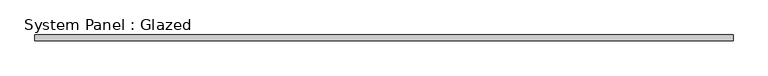
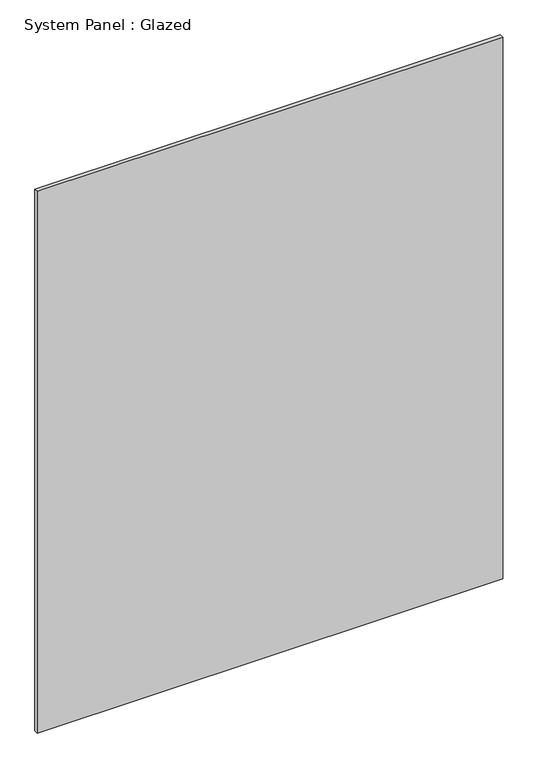
"""IFC4 building model written with IfcOpenShell, lengths in millimetres: plate geometry, System Panel : Glazed."""

from ifc_helpers import new_model, si_unit, origin, origin_with_axes, place, context, project, spatial, polyline, outline, extrude, source, transform, mapped, element, save


def system_panel_glazed_c96b3bd4(model_context):
    return source(origin(), model_context, "Body", "SweptSolid", [
        extrude(outline(polyline([(1558.4826283, 19.05), (-1558.4826283, 19.05), (-1558.4826283, 44.45), (1558.4826283, 44.45), (1558.4826283, 19.05)])), origin_with_axes(), (0.0, 0.0, 1.0), 3835.4),
    ])


if __name__ == "__main__":
    model = new_model("IFC4")
    model_context = context("Model", 3, world=origin())
    ifc_project = project(units=[si_unit("LENGTHUNIT", "METRE", prefix="MILLI")], contexts=[model_context])
    site = spatial("IfcSite", under=ifc_project)
    building = spatial("IfcBuilding", under=site)
    placement = place(None, origin())
    system_panel_glazed_shape = system_panel_glazed_c96b3bd4(model_context)
    element("IfcPlate", 1, ObjectType="System Panel : Glazed", at=placement, inside=building, context=model_context, shape_type="MappedRepresentation", body=[
        mapped(system_panel_glazed_shape, transform((0.0, 0.0, 0.0), x_axis=(1.0, 0.0, 0.0), y_axis=(0.0, 1.0, 0.0), z_axis=(0.0, 0.0, 1.0))),
    ])
    save(model, "model.ifc")

# Revit data of these elements
# Type "System Panel : Glazed"
#   Construction Type Id = "GSP4R"
#   Analytic Construction = "1/8 in Pilkington single glazing"
#   Visual Light Transmittance = 0.9
#   Solar Heat Gain Coefficient = 0.86
#   Heat Transfer Coefficient (U) = 1.18115 BTU/(h·ft²·°F)
# Element 1 (IfcPlate, "System Panel : Glazed")
#   Materials on its faces: "Glass"
# Materials
#   "Glass": class "Glass", colour RGB 0 128 192, transparency 0.75, Description = "Soda Lime Glass", Cost = 0
